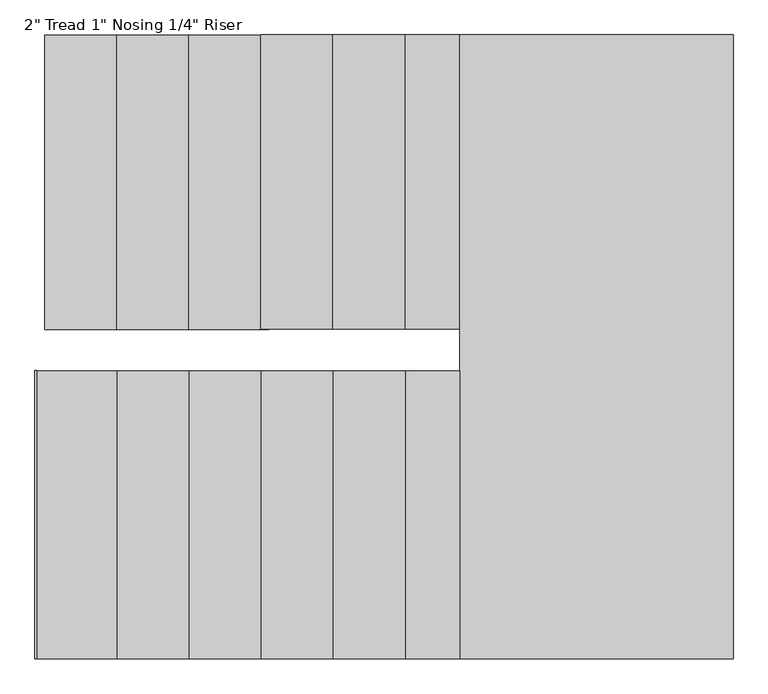
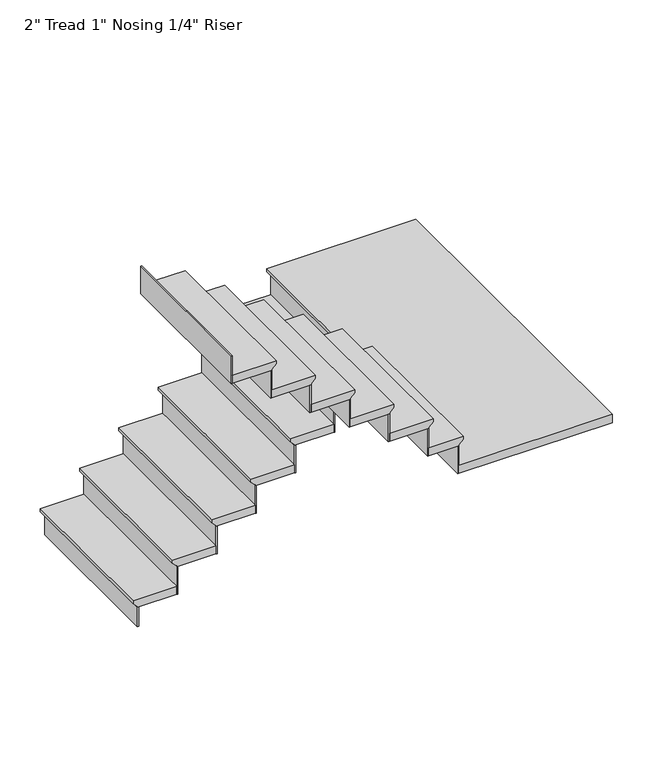
"""IFC4 building model written with IfcOpenShell, lengths in millimetres: stair flight geometry."""

from ifc_helpers import new_model, si_unit, origin, place, context, project, spatial, faceted_brep, source, transform, mapped, element, save


def stair_flight_8cfd25ce(model_context):
    return source(origin(), model_context, "Body", "Brep", [
        faceted_brep([(-1022.6415352, -3861.2539367, 9751.4833333), (-1022.6415352, -3861.2539367, 9770.5333333), (-1022.6415352, -2926.4769687, 9770.5333333), (-1022.6415352, -2926.4769687, 9751.4833333), (-997.2415352, -3861.2539367, 9726.0833333), (-997.2415352, -2926.4769687, 9726.0833333), (-768.6415352, -3861.2539367, 9770.5333333), (-768.6415352, -2926.4769687, 9770.5333333), (-997.2415352, -2926.4769687, 9719.7333333), (-768.6415352, -2926.4769687, 9719.7333333), (-768.6415352, -3861.2539367, 9719.7333333), (-997.2415352, -3861.2539367, 9719.7333333)], [[[0, 1, 2, 3]], [[4, 0, 3, 5]], [[2, 1, 6, 7]], [[8, 9, 10, 11]], [[2, 7, 9, 8, 5, 3]], [[8, 11, 4, 5]], [[6, 1, 0, 4, 11, 10]], [[7, 6, 10, 9]]]),
        faceted_brep([(-997.2415352, -3861.2539367, 9719.7333333), (-997.2415352, -3861.2539367, 9601.2), (-990.8915352, -3861.2539367, 9601.2), (-990.8915352, -3861.2539367, 9719.7333333), (-997.2415352, -2926.4769687, 9719.7333333), (-990.8915352, -2926.4769687, 9719.7333333), (-990.8915352, -2926.4769687, 9601.2), (-997.2415352, -2926.4769687, 9601.2)], [[[0, 1, 2, 3]], [[4, 5, 6, 7]], [[1, 0, 4, 7]], [[2, 1, 7, 6]], [[3, 2, 6, 5]], [[0, 3, 5, 4]]]),
        faceted_brep([(-768.6415352, -3861.2539367, 9889.0666667), (-768.6415352, -3861.2539367, 9719.7333333), (-762.2915352, -3861.2539367, 9719.7333333), (-762.2915352, -3861.2539367, 9889.0666667), (-768.6415352, -2926.4769687, 9889.0666667), (-762.2915352, -2926.4769687, 9889.0666667), (-762.2915352, -2926.4769687, 9719.7333333), (-768.6415352, -2926.4769687, 9719.7333333)], [[[0, 1, 2, 3]], [[4, 5, 6, 7]], [[1, 0, 4, 7]], [[2, 1, 7, 6]], [[3, 2, 6, 5]], [[0, 3, 5, 4]]]),
        faceted_brep([(-794.0415352, -2926.4769687, 9939.8666667), (-794.0415352, -3861.2539367, 9939.8666667), (-540.0415352, -3861.2539367, 9939.8666667), (-540.0415352, -2926.4769687, 9939.8666667), (-768.6415352, -2926.4769687, 9889.0666667), (-540.0415352, -2926.4769687, 9889.0666667), (-540.0415352, -3861.2539367, 9889.0666667), (-768.6415352, -3861.2539367, 9889.0666667), (-768.6415352, -2926.4769687, 9895.4166667), (-794.0415352, -2926.4769687, 9920.8166667), (-768.6415352, -3861.2539367, 9895.4166667), (-794.0415352, -3861.2539367, 9920.8166667)], [[[0, 1, 2, 3]], [[4, 5, 6, 7]], [[0, 3, 5, 4, 8, 9]], [[4, 7, 10, 8]], [[2, 1, 11, 10, 7, 6]], [[3, 2, 6, 5]], [[11, 1, 0, 9]], [[10, 11, 9, 8]]]),
        faceted_brep([(-540.0415352, -3861.2539367, 10058.4), (-540.0415352, -3861.2539367, 9889.0666667), (-533.6915352, -3861.2539367, 9889.0666667), (-533.6915352, -3861.2539367, 10058.4), (-540.0415352, -2926.4769687, 10058.4), (-533.6915352, -2926.4769687, 10058.4), (-533.6915352, -2926.4769687, 9889.0666667), (-540.0415352, -2926.4769687, 9889.0666667)], [[[0, 1, 2, 3]], [[4, 5, 6, 7]], [[1, 0, 4, 7]], [[2, 1, 7, 6]], [[3, 2, 6, 5]], [[0, 3, 5, 4]]]),
        faceted_brep([(-565.4415352, -2926.4769687, 10109.2), (-565.4415352, -3861.2539367, 10109.2), (-311.4415352, -3861.2539367, 10109.2), (-311.4415352, -2926.4769687, 10109.2), (-540.0415352, -2926.4769687, 10058.4), (-311.4415352, -2926.4769687, 10058.4), (-311.4415352, -3861.2539367, 10058.4), (-540.0415352, -3861.2539367, 10058.4), (-540.0415352, -2926.4769687, 10064.75), (-565.4415352, -2926.4769687, 10090.15), (-540.0415352, -3861.2539367, 10064.75), (-565.4415352, -3861.2539367, 10090.15)], [[[0, 1, 2, 3]], [[4, 5, 6, 7]], [[0, 3, 5, 4, 8, 9]], [[4, 7, 10, 8]], [[2, 1, 11, 10, 7, 6]], [[3, 2, 6, 5]], [[11, 1, 0, 9]], [[10, 11, 9, 8]]]),
        faceted_brep([(-311.4415352, -3861.2539367, 10227.7333333), (-311.4415352, -3861.2539367, 10058.4), (-305.0915352, -3861.2539367, 10058.4), (-305.0915352, -3861.2539367, 10227.7333333), (-311.4415352, -2926.4769687, 10227.7333333), (-305.0915352, -2926.4769687, 10227.7333333), (-305.0915352, -2926.4769687, 10058.4), (-311.4415352, -2926.4769687, 10058.4)], [[[0, 1, 2, 3]], [[4, 5, 6, 7]], [[1, 0, 4, 7]], [[2, 1, 7, 6]], [[3, 2, 6, 5]], [[0, 3, 5, 4]]]),
        faceted_brep([(-336.8415352, -2926.4769687, 10278.5333333), (-336.8415352, -3861.2539367, 10278.5333333), (-82.8415352, -3861.2539367, 10278.5333333), (-82.8415352, -2926.4769687, 10278.5333333), (-311.4415352, -2926.4769687, 10227.7333333), (-82.8415352, -2926.4769687, 10227.7333333), (-82.8415352, -3861.2539367, 10227.7333333), (-311.4415352, -3861.2539367, 10227.7333333), (-311.4415352, -2926.4769687, 10234.0833333), (-336.8415352, -2926.4769687, 10259.4833333), (-311.4415352, -3861.2539367, 10234.0833333), (-336.8415352, -3861.2539367, 10259.4833333)], [[[0, 1, 2, 3]], [[4, 5, 6, 7]], [[0, 3, 5, 4, 8, 9]], [[4, 7, 10, 8]], [[2, 1, 11, 10, 7, 6]], [[3, 2, 6, 5]], [[11, 1, 0, 9]], [[10, 11, 9, 8]]]),
        faceted_brep([(-82.8415352, -3861.2539367, 10397.0666667), (-82.8415352, -3861.2539367, 10227.7333333), (-76.4915352, -3861.2539367, 10227.7333333), (-76.4915352, -3861.2539367, 10397.0666667), (-82.8415352, -2926.4769687, 10397.0666667), (-76.4915352, -2926.4769687, 10397.0666667), (-76.4915352, -2926.4769687, 10227.7333333), (-82.8415352, -2926.4769687, 10227.7333333)], [[[0, 1, 2, 3]], [[4, 5, 6, 7]], [[1, 0, 4, 7]], [[2, 1, 7, 6]], [[3, 2, 6, 5]], [[0, 3, 5, 4]]]),
        faceted_brep([(-108.2415352, -2926.4769687, 10447.8666667), (-108.2415352, -3861.2539367, 10447.8666667), (145.7584648, -3861.2539367, 10447.8666667), (145.7584648, -2926.4769687, 10447.8666667), (-82.8415352, -2926.4769687, 10397.0666667), (145.7584648, -2926.4769687, 10397.0666667), (145.7584648, -3861.2539367, 10397.0666667), (-82.8415352, -3861.2539367, 10397.0666667), (-82.8415352, -2926.4769687, 10403.4166667), (-108.2415352, -2926.4769687, 10428.8166667), (-82.8415352, -3861.2539367, 10403.4166667), (-108.2415352, -3861.2539367, 10428.8166667)], [[[0, 1, 2, 3]], [[4, 5, 6, 7]], [[0, 3, 5, 4, 8, 9]], [[4, 7, 10, 8]], [[2, 1, 11, 10, 7, 6]], [[3, 2, 6, 5]], [[11, 1, 0, 9]], [[10, 11, 9, 8]]]),
        faceted_brep([(145.7584648, -3861.2539367, 10566.4), (145.7584648, -3861.2539367, 10397.0666667), (152.1084648, -3861.2539367, 10397.0666667), (152.1084648, -3861.2539367, 10566.4), (145.7584648, -2926.4769687, 10566.4), (152.1084648, -2926.4769687, 10566.4), (152.1084648, -2926.4769687, 10397.0666667), (145.7584648, -2926.4769687, 10397.0666667)], [[[0, 1, 2, 3]], [[4, 5, 6, 7]], [[1, 0, 4, 7]], [[2, 1, 7, 6]], [[3, 2, 6, 5]], [[0, 3, 5, 4]]]),
        faceted_brep([(120.3584648, -2926.4769687, 10617.2), (120.3584648, -3861.2539367, 10617.2), (320.0221038, -3861.2539367, 10617.2), (320.0221038, -2926.4769687, 10617.2), (145.7584648, -2926.4769687, 10566.4), (320.0221038, -2926.4769687, 10566.4), (320.0221038, -3861.2539367, 10566.4), (145.7584648, -3861.2539367, 10566.4), (145.7584648, -2926.4769687, 10572.75), (120.3584648, -2926.4769687, 10598.15), (145.7584648, -3861.2539367, 10572.75), (120.3584648, -3861.2539367, 10598.15)], [[[0, 1, 2, 3]], [[4, 5, 6, 7]], [[0, 3, 5, 4, 8, 9]], [[4, 7, 10, 8]], [[2, 1, 11, 10, 7, 6]], [[3, 2, 6, 5]], [[11, 1, 0, 9]], [[10, 11, 9, 8]]]),
        faceted_brep([(320.0221038, -3861.2539367, 10735.7333333), (320.0221038, -3861.2539367, 10566.4), (326.3721038, -3861.2539367, 10566.4), (326.3721038, -3861.2539367, 10735.7333333), (320.0221038, -2926.4769687, 10735.7333333), (326.3721038, -2926.4769687, 10735.7333333), (326.3721038, -2926.4769687, 10566.4), (320.0221038, -2926.4769687, 10566.4)], [[[0, 1, 2, 3]], [[4, 5, 6, 7]], [[1, 0, 4, 7]], [[2, 1, 7, 6]], [[3, 2, 6, 5]], [[0, 3, 5, 4]]]),
        faceted_brep([(269.2221038, -4907.6769687, 10786.5333333), (1161.7584648, -4907.6769687, 10786.5333333), (1161.7584648, -2926.4769687, 10786.5333333), (294.6221038, -2926.4769687, 10786.5333333), (294.6221038, -3993.2769687, 10786.5333333), (269.2221038, -3993.2769687, 10786.5333333), (1161.7584648, -4907.6769687, 10735.7333333), (269.2221038, -4907.6769687, 10735.7333333), (269.2221038, -3993.2769687, 10735.7333333), (294.6221038, -3993.2769687, 10735.7333333), (294.6221038, -3861.2539367, 10735.7333333), (320.0221038, -3861.2539367, 10735.7333333), (320.0221038, -2926.4769687, 10735.7333333), (1161.7584648, -2926.4769687, 10735.7333333), (320.0221038, -2926.4769687, 10742.0833333), (294.6221038, -2926.4769687, 10767.4833333), (320.0221038, -3861.2539367, 10742.0833333), (294.6221038, -3861.2539367, 10767.4833333)], [[[0, 1, 2, 3, 4, 5]], [[6, 7, 8, 9, 10, 11, 12, 13]], [[1, 0, 7, 6]], [[2, 1, 6, 13]], [[3, 2, 13, 12, 14, 15]], [[12, 11, 16, 14]], [[11, 10, 17, 16]], [[4, 3, 15, 17, 10, 9]], [[5, 4, 9, 8]], [[0, 5, 8, 7]], [[15, 14, 16, 17]]]),
        faceted_brep([(269.2221038, -3993.2769687, 10905.0666667), (269.2221038, -3993.2769687, 10735.7333333), (262.8721038, -3993.2769687, 10735.7333333), (262.8721038, -3993.2769687, 10905.0666667), (269.2221038, -4907.6769687, 10905.0666667), (262.8721038, -4907.6769687, 10905.0666667), (262.8721038, -4907.6769687, 10735.7333333), (269.2221038, -4907.6769687, 10735.7333333)], [[[0, 1, 2, 3]], [[4, 5, 6, 7]], [[1, 0, 4, 7]], [[2, 1, 7, 6]], [[3, 2, 6, 5]], [[0, 3, 5, 4]]]),
        faceted_brep([(294.6221038, -4907.6769687, 10955.8666667), (294.6221038, -3993.2769687, 10955.8666667), (94.9584648, -3993.2769687, 10955.8666667), (94.9584648, -4907.6769687, 10955.8666667), (269.2221038, -4907.6769687, 10905.0666667), (94.9584648, -4907.6769687, 10905.0666667), (94.9584648, -3993.2769687, 10905.0666667), (269.2221038, -3993.2769687, 10905.0666667), (269.2221038, -4907.6769687, 10911.4166667), (294.6221038, -4907.6769687, 10936.8166667), (269.2221038, -3993.2769687, 10911.4166667), (294.6221038, -3993.2769687, 10936.8166667)], [[[0, 1, 2, 3]], [[4, 5, 6, 7]], [[0, 3, 5, 4, 8, 9]], [[4, 7, 10, 8]], [[2, 1, 11, 10, 7, 6]], [[3, 2, 6, 5]], [[11, 1, 0, 9]], [[10, 11, 9, 8]]]),
        faceted_brep([(94.9584648, -3993.2769687, 11074.4), (94.9584648, -3993.2769687, 10905.0666667), (88.6084648, -3993.2769687, 10905.0666667), (88.6084648, -3993.2769687, 11074.4), (94.9584648, -4907.6769687, 11074.4), (88.6084648, -4907.6769687, 11074.4), (88.6084648, -4907.6769687, 10905.0666667), (94.9584648, -4907.6769687, 10905.0666667)], [[[0, 1, 2, 3]], [[4, 5, 6, 7]], [[1, 0, 4, 7]], [[2, 1, 7, 6]], [[3, 2, 6, 5]], [[0, 3, 5, 4]]]),
        faceted_brep([(120.3584648, -4907.6769687, 11125.2), (120.3584648, -3993.2769687, 11125.2), (-133.6415352, -3993.2769687, 11125.2), (-133.6415352, -4907.6769687, 11125.2), (94.9584648, -4907.6769687, 11074.4), (-133.6415352, -4907.6769687, 11074.4), (-133.6415352, -3993.2769687, 11074.4), (94.9584648, -3993.2769687, 11074.4), (94.9584648, -4907.6769687, 11080.75), (120.3584648, -4907.6769687, 11106.15), (94.9584648, -3993.2769687, 11080.75), (120.3584648, -3993.2769687, 11106.15)], [[[0, 1, 2, 3]], [[4, 5, 6, 7]], [[0, 3, 5, 4, 8, 9]], [[4, 7, 10, 8]], [[2, 1, 11, 10, 7, 6]], [[3, 2, 6, 5]], [[11, 1, 0, 9]], [[10, 11, 9, 8]]]),
        faceted_brep([(-133.6415352, -3993.2769687, 11243.7333333), (-133.6415352, -3993.2769687, 11074.4), (-139.9915352, -3993.2769687, 11074.4), (-139.9915352, -3993.2769687, 11243.7333333), (-133.6415352, -4907.6769687, 11243.7333333), (-139.9915352, -4907.6769687, 11243.7333333), (-139.9915352, -4907.6769687, 11074.4), (-133.6415352, -4907.6769687, 11074.4)], [[[0, 1, 2, 3]], [[4, 5, 6, 7]], [[1, 0, 4, 7]], [[2, 1, 7, 6]], [[3, 2, 6, 5]], [[0, 3, 5, 4]]]),
        faceted_brep([(-108.2415352, -4907.6769687, 11294.5333333), (-108.2415352, -3993.2769687, 11294.5333333), (-362.2415352, -3993.2769687, 11294.5333333), (-362.2415352, -4907.6769687, 11294.5333333), (-133.6415352, -4907.6769687, 11243.7333333), (-362.2415352, -4907.6769687, 11243.7333333), (-362.2415352, -3993.2769687, 11243.7333333), (-133.6415352, -3993.2769687, 11243.7333333), (-133.6415352, -4907.6769687, 11250.0833333), (-108.2415352, -4907.6769687, 11275.4833333), (-133.6415352, -3993.2769687, 11250.0833333), (-108.2415352, -3993.2769687, 11275.4833333)], [[[0, 1, 2, 3]], [[4, 5, 6, 7]], [[0, 3, 5, 4, 8, 9]], [[4, 7, 10, 8]], [[2, 1, 11, 10, 7, 6]], [[3, 2, 6, 5]], [[11, 1, 0, 9]], [[10, 11, 9, 8]]]),
        faceted_brep([(-362.2415352, -3993.2769687, 11413.0666667), (-362.2415352, -3993.2769687, 11243.7333333), (-368.5915352, -3993.2769687, 11243.7333333), (-368.5915352, -3993.2769687, 11413.0666667), (-362.2415352, -4907.6769687, 11413.0666667), (-368.5915352, -4907.6769687, 11413.0666667), (-368.5915352, -4907.6769687, 11243.7333333), (-362.2415352, -4907.6769687, 11243.7333333)], [[[0, 1, 2, 3]], [[4, 5, 6, 7]], [[1, 0, 4, 7]], [[2, 1, 7, 6]], [[3, 2, 6, 5]], [[0, 3, 5, 4]]]),
        faceted_brep([(-336.8415352, -4907.6769687, 11463.8666667), (-336.8415352, -3993.2769687, 11463.8666667), (-590.8415352, -3993.2769687, 11463.8666667), (-590.8415352, -4907.6769687, 11463.8666667), (-362.2415352, -4907.6769687, 11413.0666667), (-590.8415352, -4907.6769687, 11413.0666667), (-590.8415352, -3993.2769687, 11413.0666667), (-362.2415352, -3993.2769687, 11413.0666667), (-362.2415352, -4907.6769687, 11419.4166667), (-336.8415352, -4907.6769687, 11444.8166667), (-362.2415352, -3993.2769687, 11419.4166667), (-336.8415352, -3993.2769687, 11444.8166667)], [[[0, 1, 2, 3]], [[4, 5, 6, 7]], [[0, 3, 5, 4, 8, 9]], [[4, 7, 10, 8]], [[2, 1, 11, 10, 7, 6]], [[3, 2, 6, 5]], [[11, 1, 0, 9]], [[10, 11, 9, 8]]]),
        faceted_brep([(-590.8415352, -3993.2769687, 11582.4), (-590.8415352, -3993.2769687, 11413.0666667), (-597.1915352, -3993.2769687, 11413.0666667), (-597.1915352, -3993.2769687, 11582.4), (-590.8415352, -4907.6769687, 11582.4), (-597.1915352, -4907.6769687, 11582.4), (-597.1915352, -4907.6769687, 11413.0666667), (-590.8415352, -4907.6769687, 11413.0666667)], [[[0, 1, 2, 3]], [[4, 5, 6, 7]], [[1, 0, 4, 7]], [[2, 1, 7, 6]], [[3, 2, 6, 5]], [[0, 3, 5, 4]]]),
        faceted_brep([(-565.4415352, -4907.6769687, 11633.2), (-565.4415352, -3993.2769687, 11633.2), (-819.4415352, -3993.2769687, 11633.2), (-819.4415352, -4907.6769687, 11633.2), (-590.8415352, -4907.6769687, 11582.4), (-819.4415352, -4907.6769687, 11582.4), (-819.4415352, -3993.2769687, 11582.4), (-590.8415352, -3993.2769687, 11582.4), (-590.8415352, -4907.6769687, 11588.75), (-565.4415352, -4907.6769687, 11614.15), (-590.8415352, -3993.2769687, 11588.75), (-565.4415352, -3993.2769687, 11614.15)], [[[0, 1, 2, 3]], [[4, 5, 6, 7]], [[0, 3, 5, 4, 8, 9]], [[4, 7, 10, 8]], [[2, 1, 11, 10, 7, 6]], [[3, 2, 6, 5]], [[11, 1, 0, 9]], [[10, 11, 9, 8]]]),
        faceted_brep([(-819.4415352, -3993.2769687, 11751.7333333), (-819.4415352, -3993.2769687, 11582.4), (-825.7915352, -3993.2769687, 11582.4), (-825.7915352, -3993.2769687, 11751.7333333), (-819.4415352, -4907.6769687, 11751.7333333), (-825.7915352, -4907.6769687, 11751.7333333), (-825.7915352, -4907.6769687, 11582.4), (-819.4415352, -4907.6769687, 11582.4)], [[[0, 1, 2, 3]], [[4, 5, 6, 7]], [[1, 0, 4, 7]], [[2, 1, 7, 6]], [[3, 2, 6, 5]], [[0, 3, 5, 4]]]),
        faceted_brep([(-1048.0415352, -3993.2769687, 11921.0666667), (-1048.0415352, -3993.2769687, 11751.7333333), (-1054.3915352, -3993.2769687, 11751.7333333), (-1054.3915352, -3993.2769687, 11921.0666667), (-1048.0415352, -4907.6769687, 11921.0666667), (-1054.3915352, -4907.6769687, 11921.0666667), (-1054.3915352, -4907.6769687, 11751.7333333), (-1048.0415352, -4907.6769687, 11751.7333333)], [[[0, 1, 2, 3]], [[4, 5, 6, 7]], [[1, 0, 4, 7]], [[2, 1, 7, 6]], [[3, 2, 6, 5]], [[0, 3, 5, 4]]]),
        faceted_brep([(-794.0415352, -4907.6769687, 11802.5333333), (-794.0415352, -3993.2769687, 11802.5333333), (-1048.0415352, -3993.2769687, 11802.5333333), (-1048.0415352, -4907.6769687, 11802.5333333), (-819.4415352, -4907.6769687, 11751.7333333), (-1048.0415352, -4907.6769687, 11751.7333333), (-1048.0415352, -3993.2769687, 11751.7333333), (-819.4415352, -3993.2769687, 11751.7333333), (-819.4415352, -4907.6769687, 11758.0833333), (-794.0415352, -4907.6769687, 11783.4833333), (-819.4415352, -3993.2769687, 11758.0833333), (-794.0415352, -3993.2769687, 11783.4833333)], [[[0, 1, 2, 3]], [[4, 5, 6, 7]], [[0, 3, 5, 4, 8, 9]], [[4, 7, 10, 8]], [[2, 1, 11, 10, 7, 6]], [[3, 2, 6, 5]], [[11, 1, 0, 9]], [[10, 11, 9, 8]]]),
    ])


if __name__ == "__main__":
    model = new_model("IFC4")
    model_context = context("Model", 3, world=origin())
    ifc_project = project(units=[si_unit("LENGTHUNIT", "METRE", prefix="MILLI")], contexts=[model_context])
    site = spatial("IfcSite", under=ifc_project)
    building = spatial("IfcBuilding", under=site)
    placement = place(None, origin())
    stair_flight_shape = stair_flight_8cfd25ce(model_context)
    element("IfcStairFlight", 1, ObjectType="2\" Tread 1\" Nosing 1/4\" Riser", at=placement, inside=building, context=model_context, shape_type="MappedRepresentation", body=[
        mapped(stair_flight_shape, transform((0.0, 0.0, 0.0), x_axis=(1.0, 0.0, 0.0), y_axis=(0.0, 1.0, 0.0), z_axis=(0.0, 0.0, 1.0))),
    ])
    save(model, "model.ifc")
